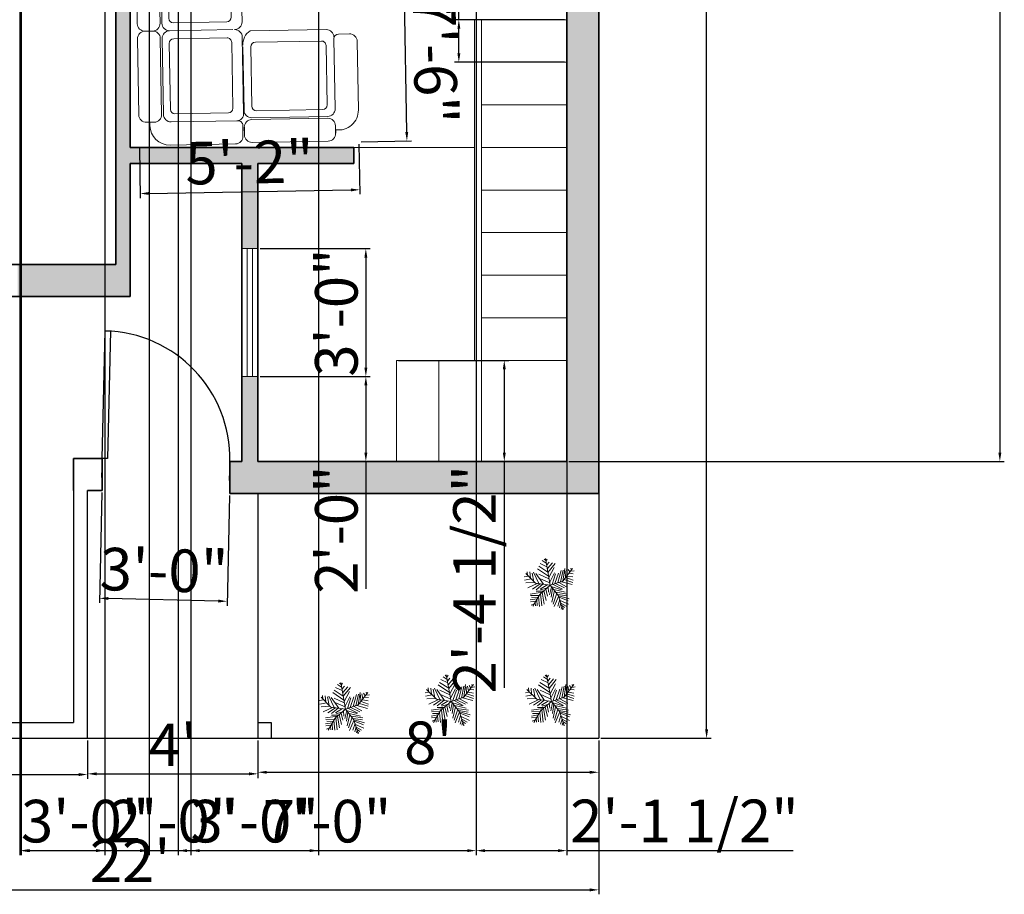
# Model space of a CAD drawing. Units: inches. Extents: x 1810 to 2254, y 313 to 1026.
# Tile 2 of 7: x 1976 to 2254, y 313 to 559. Entities that reach past the tile are written whole.
import ezdxf

# ---------------------------------------------------------------- set-up
doc = ezdxf.new("R2010")
doc.units = ezdxf.units.IN
for name, color, linetype, lineweight in [('A-ANNO-DIMS', 2, 'Continuous', 18), ('A-DOOR', 4, 'Continuous', 25), ('A-FLOR-STRS', 7, 'Continuous', 18), ('A-FURN', 8, 'Continuous', 18), ('A-GLAZ', 4, 'Continuous', 18), ('A-WALL', 7, 'Continuous', 35), ('C-SITE', 7, 'Continuous', 25), ('L-PLNT', 3, 'Continuous', 13)]:
    doc.layers.add(name, color=color, linetype=linetype, lineweight=lineweight)
doc.layers.add('A-WALL-PATT', color=252, linetype='Continuous', lineweight=13, true_color=0x939598)
doc.styles.get("Standard").update_dxf_attribs({"font": 'arial.ttf'})
doc.dimstyles.new('ISO-25', dxfattribs={"dimtxt": 12, "dimasz": 2.5, "dimexe": 1.25, "dimexo": 0.625, "dimtad": 1, "dimdec": 1, "dimlunit": 4, "dimtxsty": 'Standard', "dimcen": 2.5, "dimadec": 0, "dimazin": 0, "dimtfac": 1, "dimtdec": 1, "dimtmove": 0, "dimatfit": 3, "dimfxl": 1, "dimarcsym": 0})

# ---------------------------------------------------------------- blocks, each defined once
blk = doc.blocks.new('A$C611E44E9')
for p, q in [((0.6611, 1.4447), (0.2101, 1.4447)), ((0.7111, 1.3223), (0.7111, 1.3947)), ((0.0084, 1.2424), (0.0084, 0.7424)), ((0.1084, 1.2927), (0.0584, 1.2927)), ((0.0584, 1.2924), (0.1084, 1.2924)), ((0.1584, 1.2424), (0.1584, 0.7424)), ((0.1705, 1.2422), (0.1705, 0.7424)), ((0.6811, 1.2924), (0.2205, 1.2924)), ((0.6811, 1.2924), (0.2205, 1.2924)), ((0.6811, 1.2922), (0.2205, 1.2922)), ((0.2465, 1.2392), (0.6374, 1.2392)), ((0.7418, 0.7424), (0.7418, 1.2422)), ((0.2165, 0.7749), (0.2165, 1.2092)), ((0.6674, 1.2092), (0.6674, 0.7749)), ((0.6374, 0.7449), (0.2465, 0.7449)), ((0.1224, 0.6827), (0.05, 0.6827)), ((0.1084, 0.6927), (0.0584, 0.6927)), ((0.0584, 0.6924), (0.1084, 0.6924)), ((0.1524, 0.6527), (0.1524, 0.2121)), ((0.2024, 0.6896), (0.7021, 0.6896)), ((0.6373, 0.6924), (0.2205, 0.6924)), ((0.6373, 0.6924), (0.2205, 0.6924)), ((0.8021, 0.6896), (1.3018, 0.6896)), ((1.4021, 0.6896), (1.9018, 0.6896)), ((1.982, 0.6589), (2.0543, 0.6589)), ((0, 0.6327), (0, 0.2017)), ((0.2048, 0.5892), (0.2048, 0.2381)), ((0.6691, 0.6192), (0.2348, 0.6192)), ((0.6991, 0.2381), (0.6991, 0.5892)), ((0.7521, 0.6289), (0.7521, 0.2121)), ((0.7521, 0.6289), (0.7521, 0.2121)), ((0.8045, 0.5892), (0.8045, 0.2381)), ((1.2688, 0.6192), (0.8345, 0.6192)), ((1.2988, 0.2381), (1.2988, 0.5892)), ((1.3521, 0.6289), (1.3521, 0.2121)), ((1.3521, 0.6289), (1.3521, 0.2121)), ((1.4045, 0.5892), (1.4045, 0.2381)), ((1.8688, 0.6192), (1.4345, 0.6192)), ((1.8988, 0.2381), (1.8988, 0.5892)), ((1.9518, 0.6289), (1.9518, 0.2121)), ((1.952, 0.6289), (1.952, 0.2121)), ((2.1043, 0.6089), (2.1043, 0.2017)), ((0.2348, 0.2081), (0.6691, 0.2081)), ((0.8345, 0.2081), (1.2688, 0.2081)), ((1.4345, 0.2081), (1.8688, 0.2081)), ((0.7021, 0.1621), (0.2024, 0.1621)), ((0.7024, 0.15), (0.2024, 0.15)), ((1.3018, 0.1621), (0.8021, 0.1621)), ((1.3021, 0.15), (0.8021, 0.15)), ((1.9018, 0.1621), (1.4021, 0.1621)), ((1.9021, 0.15), (1.4021, 0.15)), ((0.13, 0.0717), (0.15, 0.0717)), ((0.1524, 0.05), (0.1524, 0.1)), ((0.7521, 0.05), (0.7521, 0.1)), ((0.7524, 0.1), (0.7524, 0.05)), ((1.3521, 0.05), (1.3521, 0.1)), ((1.3524, 0.1), (1.3524, 0.05)), ((1.952, 0.05), (1.952, 0.1)), ((1.9521, 0.1), (1.9521, 0.05)), ((1.9743, 0.0717), (1.9543, 0.0717)), ((0.7024, 0), (0.2024, 0)), ((1.3021, 0), (0.8021, 0)), ((1.9021, 0), (1.4021, 0))]:
    blk.add_line(p, q)
for centre, radius, start, end in [((0.2101, 1.3147), 0.13, 90, 189.86144), ((0.6611, 1.3947), 0.05, 0, 90), ((0.6811, 1.3223), 0.03, 270, 0), ((0.0584, 1.2424), 0.05, 90, 180), ((0.1084, 1.2424), 0.05, 0, 90), ((0.2205, 1.2422), 0.05, 90, 180), ((0.2465, 1.2092), 0.03, 90, 180), ((0.6374, 1.2092), 0.03, 0, 90), ((0.6918, 1.2422), 0.05, 0, 90), ((0.0584, 0.7424), 0.05, 180, 270), ((0.1084, 0.7424), 0.05, 270, 0), ((0.2205, 0.7424), 0.05, 180, 270), ((0.2465, 0.7749), 0.03, 180, 270), ((0.6374, 0.7749), 0.03, 270, 0), ((0.653, 0.796), 0.1037, 267.24891, 328.87945), ((0.05, 0.6327), 0.05, 90, 180), ((0.1224, 0.6527), 0.03, 0, 90), ((0.1981, 0.6441), 0.0458, 84.66489, 178.99029), ((0.7021, 0.6396), 0.05, 0, 90), ((0.8021, 0.6396), 0.05, 90, 180), ((1.3018, 0.6396), 0.05, 0, 90), ((1.4021, 0.6396), 0.05, 90, 180), ((1.9018, 0.6396), 0.05, 0, 90), ((1.982, 0.6289), 0.03, 90, 180), ((2.0543, 0.6089), 0.05, 0, 90), ((0.2348, 0.5892), 0.03, 90, 180), ((0.6691, 0.5892), 0.03, 0, 90), ((0.8345, 0.5892), 0.03, 90, 180), ((1.2688, 0.5892), 0.03, 0, 90), ((1.4345, 0.5892), 0.03, 90, 180), ((1.8688, 0.5892), 0.03, 0, 90), ((0.13, 0.2017), 0.13, 180, 270), ((0.2024, 0.2121), 0.05, 180, 270), ((0.2348, 0.2381), 0.03, 180, 270), ((0.6691, 0.2381), 0.03, 270, 0), ((0.7021, 0.2121), 0.05, 270, 0), ((0.8021, 0.2121), 0.05, 180, 270), ((0.8345, 0.2381), 0.03, 180, 270), ((1.2688, 0.2381), 0.03, 270, 0), ((1.3018, 0.2121), 0.05, 270, 0), ((1.4021, 0.2121), 0.05, 180, 270), ((1.4345, 0.2381), 0.03, 180, 270), ((1.8688, 0.2381), 0.03, 270, 0), ((1.9018, 0.2121), 0.05, 270, 0), ((1.9743, 0.2017), 0.13, 270, 0), ((0.2024, 0.1), 0.05, 90, 180), ((0.7024, 0.1), 0.05, 0, 90), ((0.8021, 0.1), 0.05, 90, 180), ((1.3021, 0.1), 0.05, 0, 90), ((1.4021, 0.1), 0.05, 90, 180), ((1.9021, 0.1), 0.05, 0, 90), ((0.2024, 0.05), 0.05, 180, 270), ((0.7024, 0.05), 0.05, 270, 0), ((0.8021, 0.05), 0.05, 180, 270), ((1.3021, 0.05), 0.05, 270, 0), ((1.4021, 0.05), 0.05, 180, 270), ((1.9021, 0.05), 0.05, 270, 0)]:
    blk.add_arc(centre, radius, start, end)
blk = doc.blocks.new('*U16')
for p, q in [((0, 0), (0, -6)), ((40, 0), (40, -6))]:
    blk.add_line(p, q)
blk.add_lwpolyline([(0, 0), (0, 40), (1.75, 40), (1.75, 0)], close=True)
blk.add_arc((0, 0), 40, 0, 90)
blk = doc.blocks.new('*U20')
for p, q in [((-7.288, 39.707), (-21.778, 46.673)), ((-8.737, 47.138), (-17.069, 52.711)), ((-10.186, 53.64), (-13.084, 55.962)), ((0, 0), (-10.5, 57)), ((-9.099, 51.782), (-6.563, 55.962)), ((-7.65, 43.423), (-2.578, 49.46)), ((-5.839, 35.992), (4.667, 48.067)), ((-5.114, 27.632), (10.463, 46.673)), ((-31.5, 4.5), (-52.5, 25.5)), ((-48.585, 21.131), (-49.309, 29.026)), ((-43.513, 28.561), (-42.427, 15.558)), ((-38.442, 26.239), (-34.819, 7.663)), ((-35.544, 28.097), (-24.314, 3.947)), ((-14.533, 2.09), (-30.834, 25.31)), ((-3.665, 19.273), (-27.574, 35.527)), ((-5.114, 28.097), (-24.676, 40.636)), ((-24.314, 23.917), (-2.941, 13.7)), ((-2.941, 16.486), (8.652, 37.85)), ((-1.129, 6.734), (9.014, 26.704)), ((3.942, 1.625), (11.187, 24.381)), ((10.101, 3.483), (17.708, 26.239)), ((16.259, 5.805), (23.142, 31.348)), ((22.055, 7.198), (27.489, 32.277)), ((27, 9), (48, 36)), ((27.127, 9.056), (31.112, 35.992)), ((31.836, 30.883), (32.561, 16.486)), ((35.096, 32.741), (37.27, 22.524)), ((38.719, 34.134), (41.979, 28.561)), ((40.53, 25.775), (48.862, 24.846)), ((43.791, 29.954), (51.036, 30.883)), ((44.153, 36.456), (45.239, 32.741)), ((-47.498, 19.737), (-55.83, 18.344)), ((-40.615, 13.7), (-55.105, 10.913)), ((-33.37, 6.269), (-52.207, 5.34)), ((-28.299, 3.483), (-47.86, -5.805)), ((-21.416, 3.018), (-38.079, -8.128)), ((0, 0), (-31.5, 4.5)), ((-15.982, 2.09), (-30.11, -9.521)), ((0, 0), (-22.5, -19.5)), ((-6.563, 1.161), (-21.416, -8.128)), ((-20.691, 13.7), (-1.129, 4.876)), ((0, 0), (27, 9)), ((0, 0), (18, -22.5)), ((6.478, 1.625), (26.04, -8.592)), ((11.187, 3.483), (30.749, -5.805)), ((18.07, 5.805), (35.096, -3.483)), ((24.229, 7.663), (46.688, 1.625)), ((29.662, 12.307), (48.137, 6.269)), ((33.285, 16.486), (48.862, 10.913)), ((36.183, 19.737), (48.137, 17.88)), ((-17.431, -15.094), (-42.789, -18.809)), ((-22.5, -19.5), (-37.5, -45)), ((-15.257, -12.772), (-30.11, -12.772)), ((-20.691, -18.345), (-17.793, -44.352)), ((-6.563, -5.805), (-19.967, -9.985)), ((-17.069, -15.094), (-12.721, -40.172)), ((-13.446, -11.378), (-8.737, -32.741)), ((-9.461, -8.592), (-6.201, -23.453)), ((-4.752, -3.483), (-3.665, -14.629)), ((2.493, -3.019), (-1.491, -20.202)), ((1.769, -2.555), (24.229, -9.521)), ((5.029, -6.27), (2.131, -25.775)), ((9.014, -11.378), (3.58, -35.992)), ((14.085, -16.951), (6.478, -40.172)), ((7.565, -9.056), (32.198, -14.629)), ((12.274, -15.094), (36.907, -18.809)), ((16.259, -19.738), (36.183, -22.989)), ((-28.299, -29.026), (-42.789, -31.348)), ((-24.314, -21.596), (-42.427, -22.06)), ((-30.834, -34.135), (-42.427, -35.528)), ((-34.457, -39.708), (-40.978, -42.494)), ((-26.849, -26.24), (-40.253, -25.775)), ((-32.646, -36.921), (-31.921, -44.352)), ((-29.023, -30.884), (-27.936, -43.887)), ((-25.038, -23.918), (-22.865, -45.281)), ((18.07, -22.524), (8.289, -45.745)), ((20.244, -30.419), (15.897, -44.816)), ((18, -22.5), (27, -52.5)), ((18.433, -22.524), (40.53, -29.026)), ((19.157, -25.311), (38.719, -33.206)), ((22.78, -37.85), (19.519, -48.532)), ((21.331, -32.741), (39.081, -40.636)), ((22.78, -38.314), (34.372, -44.816)), ((24.591, -45.745), (23.142, -50.854)), ((24.591, -43.423), (30.749, -47.603)), ((26.764, -49.925), (28.213, -50.854))]:
    blk.add_line(p, q)
blk = doc.blocks.new('*D23')
at = {"layer": 'A-ANNO-DIMS', "color": 0, "lineweight": -2, "transparency": 16777216}
for p, q in [((2130.99, 851.61), (2253.63, 851.61)), ((2252.38, 849.11), (2252.38, 437.11)), ((2130.99, 434.61), (2253.63, 434.61))]:
    blk.add_line(p, q, dxfattribs=at)
at = {"layer": 'A-ANNO-DIMS', "color": 0, "transparency": 16777216}
for points in [[(2251.96, 849.11), (2252.8, 849.11), (2252.38, 851.61)], [(2251.96, 437.11), (2252.8, 437.11), (2252.38, 434.61)]]:
    blk.add_solid(points, dxfattribs=at)
at = {"layer": 'Defpoints', "color": 0, "transparency": 16777216}
for p in [(2130.36, 851.61), (2130.36, 434.61), (2252.38, 434.61)]:
    blk.add_point(p, dxfattribs=at)
at = {"layer": 'A-ANNO-DIMS', "color": 0, "transparency": 16777216, "insert": (2245.62, 643.11), "char_height": 12, "attachment_point": 5, "rotation": 90}
blk.add_mtext('34\'-9"', dxfattribs=at)
blk = doc.blocks.new('*D26')
at = {"layer": 'A-ANNO-DIMS', "color": 0, "lineweight": -2, "transparency": 16777216}
for p, q in [((1875.36, 355.99), (1875.36, 312.66)), ((2139.36, 355.99), (2139.36, 312.66)), ((1877.86, 313.91), (2136.86, 313.91))]:
    blk.add_line(p, q, dxfattribs=at)
at = {"layer": 'A-ANNO-DIMS', "color": 0, "transparency": 16777216}
for points in [[(1877.86, 314.32), (1877.86, 313.49), (1875.36, 313.91)], [(2136.86, 314.32), (2136.86, 313.49), (2139.36, 313.91)]]:
    blk.add_solid(points, dxfattribs=at)
at = {"layer": 'Defpoints', "color": 0, "transparency": 16777216}
for p in [(1875.36, 356.61), (2139.36, 356.61), (2139.36, 313.91)]:
    blk.add_point(p, dxfattribs=at)
at = {"layer": 'A-ANNO-DIMS', "color": 0, "transparency": 16777216, "insert": (2007.36, 320.55), "char_height": 12, "attachment_point": 5}
blk.add_mtext("22'", dxfattribs=at)
blk = doc.blocks.new('*D27')
at = {"layer": 'A-ANNO-DIMS', "color": 0, "lineweight": -2, "transparency": 16777216}
for p, q in [((1875.36, 355.99), (1875.36, 345.16)), ((1995.39, 355.99), (1995.39, 345.16)), ((1877.86, 346.41), (1992.89, 346.41))]:
    blk.add_line(p, q, dxfattribs=at)
at = {"layer": 'A-ANNO-DIMS', "color": 0, "transparency": 16777216}
for points in [[(1877.86, 346.82), (1877.86, 345.99), (1875.36, 346.41)], [(1992.89, 346.82), (1992.89, 345.99), (1995.39, 346.41)]]:
    blk.add_solid(points, dxfattribs=at)
at = {"layer": 'Defpoints', "color": 0, "transparency": 16777216}
for p in [(1875.36, 356.61), (1995.39, 356.61), (1995.39, 346.41)]:
    blk.add_point(p, dxfattribs=at)
at = {"layer": 'A-ANNO-DIMS', "color": 0, "transparency": 16777216, "insert": (1935.38, 353.16), "char_height": 12, "attachment_point": 5}
blk.add_mtext("10'", dxfattribs=at)
blk = doc.blocks.new('*D28')
at = {"layer": 'A-ANNO-DIMS', "color": 0, "lineweight": -2, "transparency": 16777216}
for p, q in [((1995.39, 355.99), (1995.39, 345.35)), ((2043.36, 355.99), (2043.36, 345.35)), ((1997.89, 346.6), (2040.86, 346.6))]:
    blk.add_line(p, q, dxfattribs=at)
at = {"layer": 'A-ANNO-DIMS', "color": 0, "transparency": 16777216}
for points in [[(1997.89, 347.02), (1997.89, 346.18), (1995.39, 346.6)], [(2040.86, 347.02), (2040.86, 346.18), (2043.36, 346.6)]]:
    blk.add_solid(points, dxfattribs=at)
at = {"layer": 'Defpoints', "color": 0, "transparency": 16777216}
for p in [(1995.39, 356.61), (2043.36, 356.61), (2043.36, 346.6)]:
    blk.add_point(p, dxfattribs=at)
at = {"layer": 'A-ANNO-DIMS', "color": 0, "transparency": 16777216, "insert": (2019.38, 353.23), "char_height": 12, "attachment_point": 5}
blk.add_mtext("4'", dxfattribs=at)
blk = doc.blocks.new('*D29')
at = {"layer": 'A-ANNO-DIMS', "color": 0, "lineweight": -2, "transparency": 16777216}
for p, q in [((2043.36, 355.99), (2043.36, 345.8)), ((2139.36, 355.99), (2139.36, 345.8)), ((2045.86, 347.05), (2136.86, 347.05))]:
    blk.add_line(p, q, dxfattribs=at)
at = {"layer": 'A-ANNO-DIMS', "color": 0, "transparency": 16777216}
for points in [[(2045.86, 347.46), (2045.86, 346.63), (2043.36, 347.05)], [(2136.86, 347.46), (2136.86, 346.63), (2139.36, 347.05)]]:
    blk.add_solid(points, dxfattribs=at)
at = {"layer": 'Defpoints', "color": 0, "transparency": 16777216}
for p in [(2043.36, 356.61), (2139.36, 356.61), (2139.36, 347.05)]:
    blk.add_point(p, dxfattribs=at)
at = {"layer": 'A-ANNO-DIMS', "color": 0, "transparency": 16777216, "insert": (2091.36, 353.8), "char_height": 12, "attachment_point": 5}
blk.add_mtext("8'", dxfattribs=at)
blk = doc.blocks.new('*D44')
at = {"layer": 'A-ANNO-DIMS', "color": 0, "lineweight": -2, "transparency": 16777216}
for p, q in [((2070.88, 614.82), (2085.02, 615.06)), ((2085.29, 527.43), (2083.81, 612.54)), ((2072.44, 524.71), (2086.58, 524.96))]:
    blk.add_line(p, q, dxfattribs=at)
at = {"layer": 'A-ANNO-DIMS', "color": 0, "transparency": 16777216}
for points in [[(2084.23, 612.55), (2083.4, 612.54), (2083.77, 615.04)], [(2085.7, 527.44), (2084.87, 527.43), (2085.33, 524.93)]]:
    blk.add_solid(points, dxfattribs=at)
at = {"layer": 'Defpoints', "color": 0, "transparency": 16777216}
for p in [(2070.25, 614.81), (2083.77, 615.04), (2071.81, 524.7)]:
    blk.add_point(p, dxfattribs=at)
at = {"layer": 'A-ANNO-DIMS', "color": 0, "transparency": 16777216, "insert": (2091.38, 570.11), "char_height": 12, "attachment_point": 5, "rotation": 270.9916}
blk.add_mtext('SOFA 7\'-6"', dxfattribs=at)
blk = doc.blocks.new('*D45')
at = {"layer": 'A-ANNO-DIMS', "color": 0, "lineweight": -2, "transparency": 16777216}
for p, q in [((2009.96, 523), (2010.21, 508.86)), ((2071.82, 524.08), (2072.07, 509.93)), ((2012.68, 510.16), (2069.55, 511.14))]:
    blk.add_line(p, q, dxfattribs=at)
at = {"layer": 'A-ANNO-DIMS', "color": 0, "transparency": 16777216}
for points in [[(2012.68, 510.57), (2012.69, 509.74), (2010.18, 510.11)], [(2069.54, 511.56), (2069.55, 510.72), (2072.05, 511.18)]]:
    blk.add_solid(points, dxfattribs=at)
at = {"layer": 'Defpoints', "color": 0, "transparency": 16777216}
for p in [(2071.81, 524.7), (2009.95, 523.63), (2072.05, 511.18)]:
    blk.add_point(p, dxfattribs=at)
at = {"layer": 'A-ANNO-DIMS', "color": 0, "transparency": 16777216, "insert": (2041, 517.4), "char_height": 12, "attachment_point": 5, "rotation": 0.9916}
blk.add_mtext('5\'-2"', dxfattribs=at)
blk = doc.blocks.new('*D50')
at = {"layer": 'A-ANNO-DIMS', "color": 0, "lineweight": -2, "transparency": 16777216}
for p, q in [((2139.99, 860.61), (2171.01, 860.61)), ((2169.76, 359.11), (2169.76, 858.11)), ((2139.99, 356.61), (2171.01, 356.61))]:
    blk.add_line(p, q, dxfattribs=at)
at = {"layer": 'A-ANNO-DIMS', "color": 0, "transparency": 16777216}
for points in [[(2169.35, 858.11), (2170.18, 858.11), (2169.76, 860.61)], [(2169.35, 359.11), (2170.18, 359.11), (2169.76, 356.61)]]:
    blk.add_solid(points, dxfattribs=at)
at = {"layer": 'Defpoints', "color": 0, "transparency": 16777216}
for p in [(2139.36, 860.61), (2169.76, 860.61), (2139.36, 356.61)]:
    blk.add_point(p, dxfattribs=at)
at = {"layer": 'A-ANNO-DIMS', "color": 0, "transparency": 16777216, "insert": (2163.01, 608.61), "char_height": 12, "attachment_point": 5, "rotation": 90}
blk.add_mtext('42\'-0"', dxfattribs=at)
blk = doc.blocks.new('*D57')
at = {"layer": 'A-ANNO-DIMS', "color": 0, "lineweight": -2, "transparency": 16777216}
for p, q in [((2104.86, 718.99), (2104.86, 323.71)), ((2130.36, 718.99), (2130.36, 323.71)), ((2107.36, 324.96), (2127.86, 324.96)), ((2130.36, 324.96), (2194.18, 324.96))]:
    blk.add_line(p, q, dxfattribs=at)
at = {"layer": 'A-ANNO-DIMS', "color": 0, "transparency": 16777216}
for points in [[(2107.36, 325.38), (2107.36, 324.55), (2104.86, 324.96)], [(2127.86, 325.38), (2127.86, 324.55), (2130.36, 324.96)]]:
    blk.add_solid(points, dxfattribs=at)
at = {"layer": 'Defpoints', "color": 0, "transparency": 16777216}
for p in [(2104.86, 719.61), (2130.36, 719.61), (2130.36, 324.96)]:
    blk.add_point(p, dxfattribs=at)
at = {"layer": 'A-ANNO-DIMS', "color": 0, "transparency": 16777216, "insert": (2163.52, 331.79), "char_height": 12, "attachment_point": 5}
blk.add_mtext('2\'-1 1/2"', dxfattribs=at)
blk = doc.blocks.new('*D59')
at = {"layer": 'A-ANNO-DIMS', "color": 0, "lineweight": -2, "transparency": 16777216}
for p, q in [((2024.44, 714.49), (2024.44, 323.71)), ((2060.44, 714.49), (2060.44, 323.71)), ((2026.94, 324.96), (2057.94, 324.96))]:
    blk.add_line(p, q, dxfattribs=at)
at = {"layer": 'A-ANNO-DIMS', "color": 0, "transparency": 16777216}
for points in [[(2026.94, 325.38), (2026.94, 324.55), (2024.44, 324.96)], [(2057.94, 325.38), (2057.94, 324.55), (2060.44, 324.96)]]:
    blk.add_solid(points, dxfattribs=at)
at = {"layer": 'Defpoints', "color": 0, "transparency": 16777216}
for p in [(2024.44, 715.11), (2060.44, 715.11), (2060.44, 324.96)]:
    blk.add_point(p, dxfattribs=at)
at = {"layer": 'A-ANNO-DIMS', "color": 0, "transparency": 16777216, "insert": (2042.44, 331.72), "char_height": 12, "attachment_point": 5}
blk.add_mtext('3\'-0"', dxfattribs=at)
blk = doc.blocks.new('*D60')
at = {"layer": 'A-ANNO-DIMS', "color": 0, "lineweight": -2, "transparency": 16777216}
for p, q in [((1999.42, 425.84), (1998.69, 394.82)), ((2035.39, 424.99), (2034.66, 393.97)), ((2032.19, 395.28), (2001.22, 396.01))]:
    blk.add_line(p, q, dxfattribs=at)
at = {"layer": 'A-ANNO-DIMS', "color": 0, "transparency": 16777216}
for points in [[(2001.23, 396.43), (2001.21, 395.6), (1998.72, 396.07)], [(2032.2, 395.7), (2032.18, 394.86), (2034.69, 395.22)]]:
    blk.add_solid(points, dxfattribs=at)
at = {"layer": 'Defpoints', "color": 0, "transparency": 16777216}
for p in [(1999.44, 426.47), (2035.41, 425.61), (1998.72, 396.07)]:
    blk.add_point(p, dxfattribs=at)
at = {"layer": 'A-ANNO-DIMS', "color": 0, "transparency": 16777216, "insert": (2016.86, 402.4), "char_height": 12, "attachment_point": 5, "rotation": 358.6403}
blk.add_mtext('3\'-0"', dxfattribs=at)
blk = doc.blocks.new('*D66')
at = {"layer": 'A-ANNO-DIMS', "color": 0, "lineweight": -2, "transparency": 16777216}
for p, q in [((1976.27, 609.49), (1976.27, 323.71)), ((2000.27, 609.49), (2000.27, 323.71)), ((1978.77, 324.96), (1997.77, 324.96)), ((2000.27, 324.96), (2036.12, 324.96))]:
    blk.add_line(p, q, dxfattribs=at)
at = {"layer": 'A-ANNO-DIMS', "color": 0, "transparency": 16777216}
for points in [[(1978.77, 325.38), (1978.77, 324.55), (1976.27, 324.96)], [(1997.77, 325.38), (1997.77, 324.55), (2000.27, 324.96)]]:
    blk.add_solid(points, dxfattribs=at)
at = {"layer": 'Defpoints', "color": 0, "transparency": 16777216}
for p in [(1976.27, 610.11), (2000.27, 610.11), (2000.27, 324.96)]:
    blk.add_point(p, dxfattribs=at)
at = {"layer": 'A-ANNO-DIMS', "color": 0, "transparency": 16777216, "insert": (2019.45, 331.72), "char_height": 12, "attachment_point": 5}
blk.add_mtext('2\'-0"', dxfattribs=at)
blk = doc.blocks.new('*D67')
at = {"layer": 'A-ANNO-DIMS', "color": 0, "lineweight": -2, "transparency": 16777216}
for p, q in [((1976.68, 714.49), (1976.68, 323.71)), ((2012.68, 714.49), (2012.68, 323.71)), ((1979.18, 324.96), (2010.18, 324.96))]:
    blk.add_line(p, q, dxfattribs=at)
at = {"layer": 'A-ANNO-DIMS', "color": 0, "transparency": 16777216}
for points in [[(1979.18, 325.38), (1979.18, 324.55), (1976.68, 324.96)], [(2010.18, 325.38), (2010.18, 324.55), (2012.68, 324.96)]]:
    blk.add_solid(points, dxfattribs=at)
at = {"layer": 'Defpoints', "color": 0, "transparency": 16777216}
for p in [(1976.68, 715.11), (2012.68, 715.11), (2012.68, 324.96)]:
    blk.add_point(p, dxfattribs=at)
at = {"layer": 'A-ANNO-DIMS', "color": 0, "transparency": 16777216, "insert": (1994.68, 331.72), "char_height": 12, "attachment_point": 5}
blk.add_mtext('3\'-0"', dxfattribs=at)
blk = doc.blocks.new('*D68')
at = {"layer": 'A-ANNO-DIMS', "color": 0, "lineweight": -2, "transparency": 16777216}
for p, q in [((2020.86, 826.99), (2020.86, 323.71)), ((2104.86, 826.99), (2104.86, 323.71)), ((2023.36, 324.96), (2102.36, 324.96))]:
    blk.add_line(p, q, dxfattribs=at)
at = {"layer": 'A-ANNO-DIMS', "color": 0, "transparency": 16777216}
for points in [[(2023.36, 325.38), (2023.36, 324.55), (2020.86, 324.96)], [(2102.36, 325.38), (2102.36, 324.55), (2104.86, 324.96)]]:
    blk.add_solid(points, dxfattribs=at)
at = {"layer": 'Defpoints', "color": 0, "transparency": 16777216}
for p in [(2020.86, 827.61), (2104.86, 827.61), (2104.86, 324.96)]:
    blk.add_point(p, dxfattribs=at)
at = {"layer": 'A-ANNO-DIMS', "color": 0, "transparency": 16777216, "insert": (2062.86, 331.72), "char_height": 12, "attachment_point": 5}
blk.add_mtext('7\'-0"', dxfattribs=at)
blk = doc.blocks.new('*D70')
at = {"layer": 'A-ANNO-DIMS', "color": 0, "lineweight": -2, "transparency": 16777216}
for p, q in [((2082.99, 463.11), (2114.01, 463.11)), ((2112.76, 460.61), (2112.76, 437.11)), ((2082.99, 434.61), (2114.01, 434.61)), ((2112.76, 434.61), (2112.76, 370.8))]:
    blk.add_line(p, q, dxfattribs=at)
at = {"layer": 'A-ANNO-DIMS', "color": 0, "transparency": 16777216}
for points in [[(2112.35, 460.61), (2113.18, 460.61), (2112.76, 463.11)], [(2112.35, 437.11), (2113.18, 437.11), (2112.76, 434.61)]]:
    blk.add_solid(points, dxfattribs=at)
at = {"layer": 'Defpoints', "color": 0, "transparency": 16777216}
for p in [(2082.36, 463.11), (2082.36, 434.61), (2112.76, 434.61)]:
    blk.add_point(p, dxfattribs=at)
at = {"layer": 'A-ANNO-DIMS', "color": 0, "transparency": 16777216, "insert": (2105.93, 401.45), "char_height": 12, "attachment_point": 5, "rotation": 90}
blk.add_mtext('2\'-4 1/2"', dxfattribs=at)
blk = doc.blocks.new('*D71')
at = {"layer": 'A-ANNO-DIMS', "color": 0, "lineweight": -2, "transparency": 16777216}
for p, q in [((2043.99, 458.59), (2075.01, 458.59)), ((2073.76, 456.09), (2073.76, 437.11)), ((2043.99, 434.61), (2075.01, 434.61)), ((2073.76, 434.61), (2073.76, 398.76))]:
    blk.add_line(p, q, dxfattribs=at)
at = {"layer": 'A-ANNO-DIMS', "color": 0, "transparency": 16777216}
for points in [[(2073.35, 456.09), (2074.18, 456.09), (2073.76, 458.59)], [(2073.35, 437.11), (2074.18, 437.11), (2073.76, 434.61)]]:
    blk.add_solid(points, dxfattribs=at)
at = {"layer": 'Defpoints', "color": 0, "transparency": 16777216}
for p in [(2043.36, 458.59), (2043.36, 434.61), (2073.76, 434.61)]:
    blk.add_point(p, dxfattribs=at)
at = {"layer": 'A-ANNO-DIMS', "color": 0, "transparency": 16777216, "insert": (2067.01, 415.43), "char_height": 12, "attachment_point": 5, "rotation": 90}
blk.add_mtext('2\'-0"', dxfattribs=at)
blk = doc.blocks.new('*D74')
at = {"layer": 'A-ANNO-DIMS', "color": 0, "lineweight": -2, "transparency": 16777216}
for p, q in [((2043.99, 494.59), (2075.01, 494.59)), ((2073.76, 492.09), (2073.76, 461.09)), ((2043.99, 458.59), (2075.01, 458.59))]:
    blk.add_line(p, q, dxfattribs=at)
at = {"layer": 'A-ANNO-DIMS', "color": 0, "transparency": 16777216}
for points in [[(2073.35, 492.09), (2074.18, 492.09), (2073.76, 494.59)], [(2073.35, 461.09), (2074.18, 461.09), (2073.76, 458.59)]]:
    blk.add_solid(points, dxfattribs=at)
at = {"layer": 'Defpoints', "color": 0, "transparency": 16777216}
for p in [(2043.36, 494.59), (2043.36, 458.59), (2073.76, 458.59)]:
    blk.add_point(p, dxfattribs=at)
at = {"layer": 'A-ANNO-DIMS', "color": 0, "transparency": 16777216, "insert": (2067.01, 476.59), "char_height": 12, "attachment_point": 5, "rotation": 90}
blk.add_mtext('3\'-0"', dxfattribs=at)
blk = doc.blocks.new('*D75')
at = {"layer": 'A-ANNO-DIMS', "color": 0, "lineweight": -2, "transparency": 16777216}
for p, q in [((2099.96, 559.11), (2099.96, 593.63)), ((2129.74, 559.11), (2098.71, 559.11)), ((2099.96, 549.61), (2099.96, 556.61)), ((2129.74, 547.11), (2098.71, 547.11))]:
    blk.add_line(p, q, dxfattribs=at)
at = {"layer": 'A-ANNO-DIMS', "color": 0, "transparency": 16777216}
for points in [[(2099.55, 556.61), (2100.38, 556.61), (2099.96, 559.11)], [(2099.55, 549.61), (2100.38, 549.61), (2099.96, 547.11)]]:
    blk.add_solid(points, dxfattribs=at)
at = {"layer": 'Defpoints', "color": 0, "transparency": 16777216}
for p in [(2099.96, 559.11), (2130.36, 559.11), (2130.36, 547.11)]:
    blk.add_point(p, dxfattribs=at)
at = {"layer": 'A-ANNO-DIMS', "color": 0, "transparency": 16777216, "insert": (2093.21, 577.62), "char_height": 12, "attachment_point": 5, "rotation": 90}
blk.add_mtext('1\'-0"', dxfattribs=at)

msp = doc.modelspace()

# ---------------------------------------------------------------- hatches: boundary and pattern name
at = {"layer": 'A-WALL-PATT'}
h = msp.add_hatch(color=256, dxfattribs=at)
h.dxf.hatch_style = 1
h.paths.add_polyline_path([(1943.78, 860.61), (1875.36, 860.61), (1875.36, 706.11), (1884.36, 706.11), (1884.36, 715.11), (1968.36, 715.11), (1968.36, 703.36), (1971.96, 703.36), (1972.86, 703.36), (1972.86, 715.11), (1976.68, 715.11), (1976.68, 719.61), (1884.36, 719.61), (1884.36, 851.61), (1943.73, 851.61)])
h.paths.add_polyline_path([(2048.15, 860.61), (1979.78, 860.61), (1979.73, 851.61), (2016.36, 851.61), (2016.36, 719.61), (2012.68, 719.61), (2012.68, 716.01), (2012.68, 715.11), (2024.44, 715.11), (2024.44, 719.61), (2020.86, 719.61), (2020.86, 851.61), (2048.15, 851.61)])
h.paths.add_polyline_path([(2139.36, 860.61), (2084.15, 860.61), (2084.15, 851.61), (2130.36, 851.61), (2130.36, 719.61), (2060.44, 719.61), (2060.44, 716.01), (2060.44, 715.11), (2130.36, 715.11), (2130.36, 673.52), (2139.36, 673.52)])
h.paths.add_polyline_path([(1884.36, 682.11), (1875.36, 682.11), (1875.36, 654.79), (1884.36, 654.79), (1884.36, 662.61), (1968.36, 662.61), (1968.36, 647.42), (1971.96, 647.42), (1972.86, 647.42), (1972.86, 679.36), (1968.36, 679.36), (1968.36, 667.11), (1884.36, 667.11)])
h.paths.add_polyline_path([(1884.36, 610.11), (1972.86, 610.11), (1976.27, 610.11), (1976.27, 614.61), (1972.86, 614.61), (1972.86, 623.42), (1968.36, 623.42), (1968.36, 614.61), (1884.36, 614.61), (1884.36, 630.79), (1875.36, 630.79), (1875.36, 481.11), (1939.68, 481.11), (1939.68, 490.11), (1884.36, 490.11)])
h.paths.add_polyline_path([(2007.36, 518.61), (2038.86, 518.61), (2038.86, 494.59), (2043.36, 494.59), (2043.36, 518.61), (2070.36, 518.61), (2070.36, 523.11), (2007.36, 523.11), (2007.36, 614.61), (2000.27, 614.61), (2000.27, 610.11), (2003.36, 610.11), (2003.36, 490.11), (1975.68, 490.11), (1975.68, 481.11), (2007.36, 481.11)])
h.paths.add_polyline_path([(2139.36, 637.52), (2130.36, 637.52), (2130.36, 434.61), (2043.36, 434.61), (2043.36, 458.59), (2038.86, 458.59), (2038.86, 434.61), (2035.41, 434.61), (2035.41, 431.01), (2035.41, 425.61), (2139.36, 425.61)])

# ---------------------------------------------------------------- linework, layer by layer
at = {"layer": 'A-FLOR-STRS'}
for p, q in [((2104.36, 559.11), (2130.36, 559.11)), ((2104.36, 559.11), (2104.36, 463.11)), ((2106.36, 559.11), (2106.36, 434.61)), ((2106.36, 547.11), (2130.36, 547.11)), ((2106.36, 535.11), (2130.36, 535.11)), ((2070.36, 523.11), (2104.36, 523.11)), ((2106.36, 523.11), (2130.36, 523.11)), ((2106.36, 511.11), (2130.36, 511.11)), ((2106.36, 499.11), (2130.36, 499.11)), ((2106.36, 487.11), (2130.36, 487.11)), ((2106.36, 475.11), (2130.36, 475.11)), ((2082.36, 463.11), (2082.36, 434.61)), ((2106.36, 463.11), (2082.36, 463.11)), ((2094.36, 463.11), (2094.36, 434.61)), ((2106.36, 463.11), (2130.36, 463.11))]:
    msp.add_line(p, q, dxfattribs=at)
at = {"layer": 'A-GLAZ'}
for p, q in [((2038.86, 494.59), (2043.36, 494.59)), ((2040.36, 494.59), (2040.36, 458.59)), ((2041.86, 494.59), (2041.86, 458.59)), ((2038.86, 458.59), (2043.36, 458.59))]:
    msp.add_line(p, q, dxfattribs=at)
at = {"layer": 'A-WALL'}
for p, q in [((2139.36, 860.61), (2139.36, 425.61)), ((2130.36, 715.11), (2130.36, 434.61)), ((2007.36, 614.61), (2007.36, 523.11)), ((2003.36, 610.11), (2003.36, 490.11)), ((2007.36, 523.11), (2070.36, 523.11)), ((2070.36, 523.11), (2070.36, 518.61)), ((2007.36, 518.61), (2038.86, 518.61)), ((2007.36, 518.61), (2007.36, 481.11)), ((2038.86, 518.61), (2038.86, 434.61)), ((2043.36, 518.61), (2043.36, 434.61)), ((2043.36, 518.61), (2070.36, 518.61)), ((1884.36, 490.11), (2003.36, 490.11)), ((1875.36, 481.11), (2007.36, 481.11)), ((1991.39, 435.47), (1995.39, 435.47)), ((1991.39, 435.47), (1991.39, 426.47)), ((1995.39, 435.47), (1999.44, 435.47)), ((1999.44, 435.47), (1999.44, 426.47)), ((2035.41, 434.61), (2038.86, 434.61)), ((2035.41, 434.61), (2035.41, 425.61)), ((2043.36, 434.61), (2130.36, 434.61)), ((1995.39, 426.47), (1999.44, 426.47)), ((2035.41, 425.61), (2139.36, 425.61))]:
    msp.add_line(p, q, dxfattribs=at)
at = {"layer": 'C-SITE'}
for p, q in [((1991.39, 426.47), (1991.39, 361.11)), ((1995.39, 356.61), (1995.39, 426.47)), ((2043.36, 425.61), (2043.36, 356.61)), ((2139.36, 425.61), (2139.36, 356.61)), ((1875.36, 361.11), (1991.39, 361.11)), ((2043.36, 361.11), (2047.05, 361.11)), ((2047.05, 361.11), (2047.05, 356.61)), ((1875.36, 356.61), (1995.39, 356.61)), ((1995.39, 356.61), (2139.36, 356.61))]:
    msp.add_line(p, q, dxfattribs=at)

# ---------------------------------------------------------------- block references
at = {"layer": 'A-DOOR', "xscale": 0.899493010506624, "yscale": 0.899493010506624, "zscale": 0.899493010506624, "rotation": 358.6402788789151}
msp.add_blockref('*U16', (1999.44, 435.47), dxfattribs=at)
at = {"layer": 'A-FURN', "xscale": -42.82681931732404, "yscale": 42.82681931732404, "zscale": 42.82681931732404, "rotation": 270.9915511878509}
msp.add_blockref('A$C611E44E9', (2009.95, 523.63), dxfattribs=at)
at = {"layer": 'L-PLNT', "xscale": 0.1315167805911133, "yscale": 0.1315167805911133, "zscale": 0.1315167805911133}
for p in [(2125.71, 399.74), (2097.79, 367.02), (2126.04, 367.02), (2068.05, 364.82)]:
    msp.add_blockref('*U20', p, dxfattribs=at)

# ---------------------------------------------------------------- dimensions: what is measured, and where the dimension line sits
at = {"layer": 'A-ANNO-DIMS'}
for base, p1, p2, angle, override, picture, middle in [((2169.76, 860.61), (2139.36, 356.61), (2139.36, 860.61), 90, {"dimdec": 1, "dimlfac": 1, "dimrnd": 0, "dimzin": 1, "dimdsep": 46, "dimlunit": 4, "dimfrac": 2}, '*D50', (2163.01, 608.61)), ((2252.38, 434.61), (2130.36, 851.61), (2130.36, 434.61), 90, {"dimclrd": 0, "dimclre": 0, "dimclrt": 0}, '*D23', (2245.62, 643.11)), ((2099.96, 559.11), (2130.36, 547.11), (2130.36, 559.11), 90, {"dimdec": 1, "dimlfac": 1, "dimrnd": 0, "dimzin": 1, "dimdsep": 46, "dimlunit": 4, "dimfrac": 2}, '*D75', (2093.21, 577.62)), ((2072.05, 511.18), (2009.95, 523.63), (2071.81, 524.7), 0.9916, {"dimdec": 1, "dimlfac": 1, "dimrnd": 0, "dimzin": 1, "dimdsep": 46, "dimlunit": 4, "dimfrac": 2}, '*D45', (2041, 517.4)), ((2073.76, 458.59), (2043.36, 494.59), (2043.36, 458.59), 270, {"dimdec": 1, "dimlfac": 1, "dimrnd": 0, "dimzin": 1, "dimdsep": 46, "dimlunit": 4, "dimfrac": 2}, '*D74', (2067.01, 476.59)), ((2112.76, 434.61), (2082.36, 463.11), (2082.36, 434.61), 270, {"dimdec": 1, "dimlfac": 1, "dimrnd": 0, "dimzin": 1, "dimdsep": 46, "dimlunit": 4, "dimfrac": 2}, '*D70', (2105.93, 401.45)), ((2073.76, 434.61), (2043.36, 458.59), (2043.36, 434.61), 270, {"dimdec": 1, "dimlfac": 1, "dimrnd": 0, "dimzin": 1, "dimdsep": 46, "dimlunit": 4, "dimfrac": 2}, '*D71', (2067.01, 415.43)), ((1998.72, 396.07), (2035.41, 425.61), (1999.44, 426.47), 178.6403, {"dimdec": 1, "dimlfac": 1, "dimrnd": 0, "dimzin": 1, "dimdsep": 46, "dimlunit": 4, "dimfrac": 2}, '*D60', (2016.86, 402.4))]:
    dim = msp.add_linear_dim(base=base, p1=p1, p2=p2, angle=angle, dimstyle='ISO-25', override=override, dxfattribs=at)
    dim.commit()
    dim.dimension.update_dxf_attribs({"geometry": picture, "text_midpoint": middle})
for base, p1, p2, override, picture, middle in [((2104.86, 324.96), (2020.86, 827.61), (2104.86, 827.61), {"dimdec": 1, "dimlfac": 1, "dimrnd": 0, "dimzin": 1, "dimdsep": 46, "dimlunit": 4, "dimfrac": 2}, '*D68', (2062.86, 331.72)), ((2130.36, 324.96), (2104.86, 719.61), (2130.36, 719.61), {"dimdec": 1, "dimlfac": 1, "dimrnd": 0, "dimzin": 1, "dimdsep": 46, "dimlunit": 4, "dimfrac": 2}, '*D57', (2163.52, 331.79)), ((2012.68, 324.96), (1976.68, 715.11), (2012.68, 715.11), {"dimdec": 1, "dimlfac": 1, "dimrnd": 0, "dimzin": 1, "dimdsep": 46, "dimlunit": 4, "dimfrac": 2}, '*D67', (1994.68, 331.72)), ((2060.44, 324.96), (2024.44, 715.11), (2060.44, 715.11), {"dimdec": 1, "dimlfac": 1, "dimrnd": 0, "dimzin": 1, "dimdsep": 46, "dimlunit": 4, "dimfrac": 2}, '*D59', (2042.44, 331.72)), ((2000.27, 324.96), (1976.27, 610.11), (2000.27, 610.11), {"dimdec": 1, "dimlfac": 1, "dimrnd": 0, "dimzin": 1, "dimdsep": 46, "dimlunit": 4, "dimfrac": 2}, '*D66', (2019.45, 331.72)), ((1995.39, 346.41), (1875.36, 356.61), (1995.39, 356.61), {"dimclrd": 0, "dimclre": 0, "dimclrt": 0}, '*D27', (1935.38, 353.16)), ((2043.36, 346.6), (1995.39, 356.61), (2043.36, 356.61), {"dimclrd": 0, "dimclre": 0, "dimclrt": 0}, '*D28', (2019.38, 353.23)), ((2139.36, 347.05), (2043.36, 356.61), (2139.36, 356.61), {"dimclrd": 0, "dimclre": 0, "dimclrt": 0}, '*D29', (2091.36, 353.8)), ((2139.36, 313.91), (1875.36, 356.61), (2139.36, 356.61), {"dimclrd": 0, "dimclre": 0, "dimclrt": 0}, '*D26', (2007.36, 320.55))]:
    dim = msp.add_linear_dim(base=base, p1=p1, p2=p2, dimstyle='ISO-25', override=override, dxfattribs=at)
    dim.commit()
    dim.dimension.update_dxf_attribs({"geometry": picture, "text_midpoint": middle})
dim = msp.add_linear_dim(base=(2083.77, 615.04), p1=(2071.81, 524.7), p2=(2070.25, 614.81), angle=90.9916, text='SOFA <>', dimstyle='ISO-25', override={"dimdec": 1, "dimlfac": 1, "dimrnd": 0, "dimzin": 1, "dimdsep": 46, "dimlunit": 4, "dimfrac": 2}, dxfattribs=at)
dim.commit()
dim.dimension.update_dxf_attribs({"geometry": '*D44', "text_midpoint": (2091.38, 570.11)})

doc.saveas('drawing.dxf')
